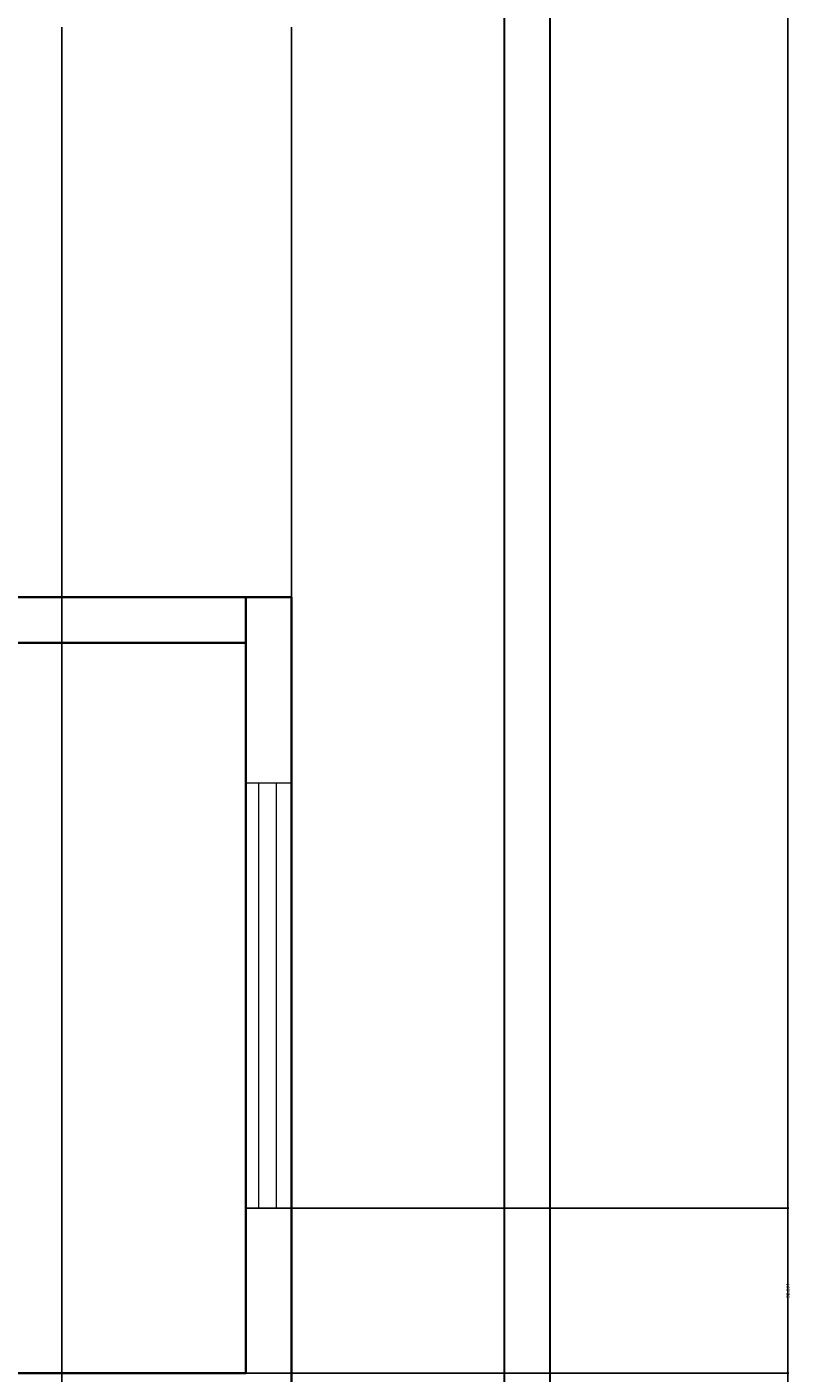
# Model space of a CAD drawing. Units: inches. Extents: x 867 to 1667, y -234 to 788.
# Tile 25 of 42: x 1517 to 1667, y -8 to 258. Entities that reach past the tile are written whole.
import ezdxf

# ---------------------------------------------------------------- set-up
doc = ezdxf.new("R2010")
doc.units = ezdxf.units.IN
doc.header["$MEASUREMENT"] = 0
for name, color, linetype, lineweight in [('A-ANNO-DIMS', 2, 'Continuous', 18), ('A-Glaz', 92, 'Continuous', 18), ('A-Wall', 7, 'Continuous', 35), ('A-WALL-SITE', 8, 'Continuous', 30)]:
    doc.layers.add(name, color=color, linetype=linetype, lineweight=lineweight)
doc.styles.get("Standard").update_dxf_attribs({"font": 'arial.ttf'})
doc.dimstyles.get("Standard").update_dxf_attribs({"dimtxt": 0.6875, "dimasz": 0.18, "dimexe": 0.18, "dimexo": 0.0625, "dimgap": 0.09, "dimtad": 0, "dimdec": 4, "dimzin": 0, "dimdsep": 46, "dimlunit": 4, "dimtxsty": 'Standard', "dimcen": 0.09, "dimadec": 0, "dimazin": 0, "dimtfac": 1, "dimtdec": 4, "dimtofl": 0, "dimtmove": 0, "dimatfit": 3, "dimfxl": 1, "dimtolj": 1, "dimtzin": 0, "dimarcsym": 0})

# ---------------------------------------------------------------- blocks, each defined once
blk = doc.blocks.new('WIN-83_90IN')
for p, q in [((0, 83.9), (9, 83.9)), ((2.51, 83.9), (2.51, 0)), ((6.08, 0), (6.08, 83.9)), ((0, 0), (9, 0))]:
    blk.add_line(p, q)
blk = doc.blocks.new('*D18')
at = {"layer": 'A-ANNO-DIMS', "color": 0, "lineweight": -2, "transparency": 16777216}
for p, q in [((1619.95, 740.62), (1667.02, 740.62)), ((1666.84, 740.44), (1666.84, 277.95)), ((1666.84, -186.23), (1666.84, 276.25)), ((1619.95, -186.41), (1667.02, -186.41))]:
    blk.add_line(p, q, dxfattribs=at)
at = {"layer": 'A-ANNO-DIMS', "color": 0, "transparency": 16777216}
for points in [[(1666.81, 740.44), (1666.87, 740.44), (1666.84, 740.62)], [(1666.81, -186.23), (1666.87, -186.23), (1666.84, -186.41)]]:
    blk.add_solid(points, dxfattribs=at)
at = {"layer": 'Defpoints', "color": 0, "transparency": 16777216}
for p in [(1619.89, 740.62), (1666.84, 740.62), (1619.89, -186.41)]:
    blk.add_point(p, dxfattribs=at)
at = {"layer": 'A-ANNO-DIMS', "color": 0, "transparency": 16777216, "insert": (1666.84, 277.1), "char_height": 0.688, "attachment_point": 5, "rotation": 90}
blk.add_mtext('\\A1;927', dxfattribs=at)
blk = doc.blocks.new('*D55')
at = {"layer": 'A-ANNO-DIMS', "color": 0, "lineweight": -2, "transparency": 16777216}
for p, q in [((1523.6, 257.55), (1523.6, -233.54)), ((1568.89, 257.55), (1568.89, -233.54)), ((1523.78, -233.36), (1544.71, -233.36)), ((1568.71, -233.36), (1547.78, -233.36))]:
    blk.add_line(p, q, dxfattribs=at)
at = {"layer": 'A-ANNO-DIMS', "color": 0, "transparency": 16777216}
for points in [[(1523.78, -233.33), (1523.78, -233.39), (1523.6, -233.36)], [(1568.71, -233.33), (1568.71, -233.39), (1568.89, -233.36)]]:
    blk.add_solid(points, dxfattribs=at)
at = {"layer": 'Defpoints', "color": 0, "transparency": 16777216}
for p in [(1523.6, 257.62), (1568.89, 257.62), (1568.89, -233.36)]:
    blk.add_point(p, dxfattribs=at)
at = {"layer": 'A-ANNO-DIMS', "color": 0, "transparency": 16777216, "insert": (1546.24, -233.36), "char_height": 0.688, "attachment_point": 5}
blk.add_mtext('\\A1;45.285', dxfattribs=at)
blk = doc.blocks.new('*D59')
at = {"layer": 'A-ANNO-DIMS', "color": 0, "lineweight": -2, "transparency": 16777216}
for p, q in [((1559.95, 24.65), (1667.02, 24.65)), ((1666.84, 24.47), (1666.84, 9.9)), ((1666.84, -7.7), (1666.84, 6.87)), ((1559.95, -7.88), (1667.02, -7.88))]:
    blk.add_line(p, q, dxfattribs=at)
at = {"layer": 'A-ANNO-DIMS', "color": 0, "transparency": 16777216}
for points in [[(1666.81, 24.47), (1666.87, 24.47), (1666.84, 24.65)], [(1666.81, -7.7), (1666.87, -7.7), (1666.84, -7.88)]]:
    blk.add_solid(points, dxfattribs=at)
at = {"layer": 'Defpoints', "color": 0, "transparency": 16777216}
for p in [(1559.89, 24.65), (1666.84, 24.65), (1559.89, -7.88)]:
    blk.add_point(p, dxfattribs=at)
at = {"layer": 'A-ANNO-DIMS', "color": 0, "transparency": 16777216, "insert": (1666.84, 8.38), "char_height": 0.688, "attachment_point": 5, "rotation": 90}
blk.add_mtext('\\A1;32.534', dxfattribs=at)

msp = doc.modelspace()

# ---------------------------------------------------------------- linework, layer by layer
at = {"layer": 'A-Wall'}
for p, q in [((1568.8866, 145.117), (1439.8866, 145.117)), ((1559.8866, 145.117), (1559.8866, -7.883)), ((1568.8866, 145.117), (1568.8866, -55.9081)), ((1559.8866, 136.117), (1439.8866, 136.117)), ((1559.8866, -7.883), (1403.8866, -7.883))]:
    msp.add_line(p, q, dxfattribs=at)
at = {"layer": 'A-WALL-SITE'}
for p, q in [((1610.8866, 740.617), (1610.8866, -186.4081)), ((1619.8866, 740.617), (1619.8866, -186.4081))]:
    msp.add_line(p, q, dxfattribs=at)

# ---------------------------------------------------------------- block references
at = {"layer": 'A-Glaz'}
msp.add_blockref('WIN-83_90IN', (1559.887, 24.651), dxfattribs=at)

# ---------------------------------------------------------------- dimensions: what is measured, and where the dimension line sits
at = {"layer": 'A-ANNO-DIMS'}
for base, p1, p2, override, picture, middle in [((1666.8366, 740.617), (1619.8866, -186.4081), (1619.8866, 740.617), {"dimdec": 0, "dimlfac": 1, "dimrnd": 0, "dimzin": 0, "dimdsep": 46, "dimlunit": 2}, '*D18', (1666.8366, 277.1045)), ((1666.8366, 24.6511), (1559.8866, -7.883), (1559.8866, 24.6511), {"dimdec": 3, "dimlfac": 1, "dimrnd": 0, "dimzin": 0, "dimdsep": 46, "dimlunit": 2}, '*D59', (1666.8366, 8.3841))]:
    dim = msp.add_linear_dim(base=base, p1=p1, p2=p2, angle=90, dimstyle='Standard', override=override, dxfattribs=at)
    dim.commit()
    dim.dimension.update_dxf_attribs({"geometry": picture, "text_midpoint": middle})
dim = msp.add_linear_dim(base=(1568.8866, -233.3581), p1=(1523.6015, 257.617), p2=(1568.8866, 257.617), dimstyle='Standard', override={"dimdec": 3, "dimlfac": 1, "dimrnd": 0, "dimzin": 0, "dimdsep": 46, "dimlunit": 2}, dxfattribs=at)
dim.commit()
dim.dimension.update_dxf_attribs({"geometry": '*D55', "text_midpoint": (1546.2441, -233.3581)})

doc.saveas('drawing.dxf')
